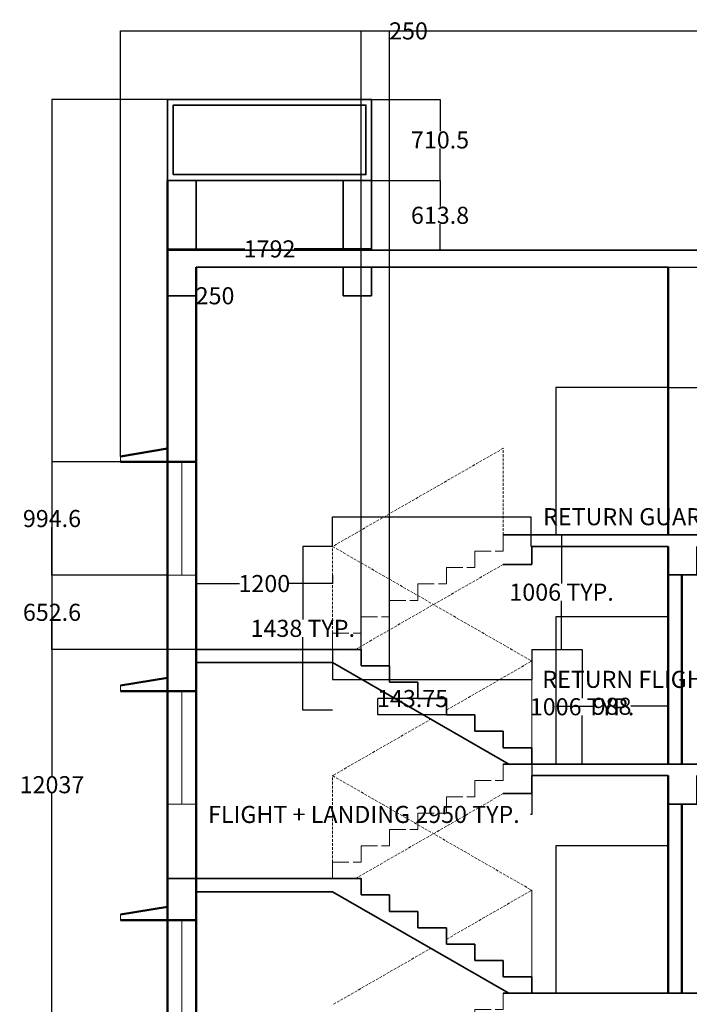
# Model space of a CAD drawing. Units: millimetres. Extents: x -1193 to 12449, y -949 to 12489.
# Tile 1 of 2: x -1193 to 4692, y 3842 to 12489. Entities that reach past the tile are written whole.
import ezdxf

# ---------------------------------------------------------------- set-up
doc = ezdxf.new("R2010")
doc.units = ezdxf.units.MM
doc.header["$LTSCALE"] = 12
doc.header["$MEASUREMENT"] = 0
doc.linetypes.add('ACAD_ISO02W100', pattern=[15, 12, -3])
doc.linetypes.add('HIDDEN', pattern=[0.375, 0.25, -0.125])
for name, color, linetype, lineweight in [('A-ANNO-DIMS', 2, 'Continuous', 18), ('A-DOOR', 3, 'Continuous', 25), ('A-FLOR', 7, 'Continuous', 35), ('A-FLOR-HRAL-BYND', 8, 'ACAD_ISO02W100', 18), ('A-FLOR-HRAL-HIDN', 8, 'HIDDEN', 18), ('A-FLOR-STRS', 7, 'Continuous', 35), ('A-FLOR-STRS-BYND', 8, 'ACAD_ISO02W100', 18), ('A-FLOR-STRS-HIDN', 8, 'HIDDEN', 18), ('A-GLAZ', 4, 'Continuous', 18), ('A-ROOF', 7, 'Continuous', 35), ('A-WALL', 7, 'Continuous', 50), ('A-WALL-BYND', 8, 'ACAD_ISO02W100', 18), ('S-BEAM', 1, 'Continuous', 35)]:
    doc.layers.add(name, color=color, linetype=linetype, lineweight=lineweight)
doc.styles.get("Standard").update_dxf_attribs({"font": 'arial.ttf'})
doc.dimstyles.get("Standard").update_dxf_attribs({"dimtxt": 150, "dimasz": 0.18, "dimexe": 0.18, "dimexo": 0.0625, "dimgap": 0.09, "dimtad": 0, "dimtih": 1, "dimtoh": 1, "dimdec": 0, "dimzin": 0, "dimdsep": 46, "dimtxsty": 'Standard', "dimcen": 0.09, "dimadec": 0, "dimazin": 0, "dimtfac": 1, "dimtdec": 0, "dimtofl": 0, "dimtmove": 0, "dimatfit": 3, "dimfxl": 1, "dimtolj": 1, "dimtzin": 0, "dimarcsym": 0})

# ---------------------------------------------------------------- blocks, each defined once
blk = doc.blocks.new('*D1')
at = {"layer": 'A-ANNO-DIMS', "color": 0, "lineweight": -2, "ltscale": 8, "transparency": 16777216}
for p, q in [((357.0112971154486, 7610.496564102366), (357.0112971154486, 7536.691782342278)), ((1557.011297115449, 7610.496564102368), (1557.011297115449, 7536.691782342278)), ((357.1912971154485, 7536.871782342278), (740.2603148507828, 7536.871782342278)), ((1556.831297115448, 7536.871782342278), (1173.762279380114, 7536.871782342278))]:
    blk.add_line(p, q, dxfattribs=at)
at = {"layer": 'A-ANNO-DIMS', "color": 0, "ltscale": 8, "transparency": 16777216}
for points in [[(357.1912971154485, 7536.901782342278), (357.1912971154485, 7536.841782342277), (357.0112971154486, 7536.871782342278)], [(1556.831297115448, 7536.901782342278), (1556.831297115448, 7536.841782342277), (1557.011297115449, 7536.871782342278)]]:
    blk.add_solid(points, dxfattribs=at)
at = {"layer": 'Defpoints', "color": 0, "ltscale": 8, "transparency": 16777216}
for p in [(357.0112971154486, 7610.559064102368), (1557.011297115449, 7610.559064102368), (1557.011297115449, 7536.871782342278)]:
    blk.add_point(p, dxfattribs=at)
at = {"layer": 'A-ANNO-DIMS', "color": 0, "ltscale": 8, "transparency": 16777216, "insert": (957.0112971154484, 7536.871782342278), "char_height": 150, "attachment_point": 5}
blk.add_mtext('\\A1;1200', dxfattribs=at)
blk = doc.blocks.new('*D2')
at = {"layer": 'A-ANNO-DIMS', "color": 0, "lineweight": -2, "ltscale": 8, "transparency": 16777216}
for p, q in [((3519.003756800259, 6598.667868016852), (3519.003756800259, 6459.014847604733)), ((4507.011297115449, 6598.667868016852), (4507.011297115449, 6459.014847604733)), ((3519.183756800259, 6459.194847604734), (3847.058045375316, 6459.194847604734)), ((4506.831297115448, 6459.194847604734), (4178.957008540391, 6459.194847604734))]:
    blk.add_line(p, q, dxfattribs=at)
at = {"layer": 'A-ANNO-DIMS', "color": 0, "ltscale": 8, "transparency": 16777216}
for points in [[(3519.183756800259, 6459.224847604733), (3519.183756800259, 6459.164847604732), (3519.003756800259, 6459.194847604734)], [(4506.831297115448, 6459.224847604733), (4506.831297115448, 6459.164847604732), (4507.011297115449, 6459.194847604734)]]:
    blk.add_solid(points, dxfattribs=at)
at = {"layer": 'Defpoints', "color": 0, "ltscale": 8, "transparency": 16777216}
for p in [(3519.003756800259, 6598.730368016852), (4507.011297115449, 6598.730368016852), (4507.011297115449, 6459.194847604734)]:
    blk.add_point(p, dxfattribs=at)
at = {"layer": 'A-ANNO-DIMS', "color": 0, "ltscale": 8, "transparency": 16777216, "insert": (4013.007526957854, 6459.194847604734), "char_height": 150, "attachment_point": 5}
blk.add_mtext('\\A1;988', dxfattribs=at)
blk = doc.blocks.new('*D6')
at = {"layer": 'A-ANNO-DIMS', "color": 0, "lineweight": -2, "ltscale": 8, "transparency": 16777216}
for p, q in [((107.0112971154485, 10064.31189252442), (107.0112971154485, 10064.42939252442)), ((107.1912971154485, 10064.24939252442), (356.8312971154485, 10064.24939252442)), ((357.0112971154486, 10064.31189252442), (357.0112971154486, 10064.42939252442)), ((357.0112971154486, 10064.24939252442), (357.1912971154486, 10064.24939252442))]:
    blk.add_line(p, q, dxfattribs=at)
at = {"layer": 'A-ANNO-DIMS', "color": 0, "ltscale": 8, "transparency": 16777216}
for points in [[(107.1912971154485, 10064.27939252442), (107.1912971154485, 10064.21939252442), (107.0112971154485, 10064.24939252442)], [(356.8312971154485, 10064.27939252442), (356.8312971154485, 10064.21939252442), (357.0112971154486, 10064.24939252442)]]:
    blk.add_solid(points, dxfattribs=at)
at = {"layer": 'Defpoints', "color": 0, "ltscale": 8, "transparency": 16777216}
for p in [(107.0112971154485, 10064.24939252442), (357.0112971154486, 10064.24939252442), (357.0112971154486, 10064.24939252442)]:
    blk.add_point(p, dxfattribs=at)
at = {"layer": 'A-ANNO-DIMS', "color": 0, "ltscale": 8, "transparency": 16777216, "insert": (524.0104922041252, 10064.24939252442), "char_height": 150, "attachment_point": 5}
blk.add_mtext('\\A1;250', dxfattribs=at)
blk = doc.blocks.new('*D7')
at = {"layer": 'A-ANNO-DIMS', "color": 0, "lineweight": -2, "ltscale": 8, "transparency": 16777216}
for p, q in [((4507.073797115451, 10464.24939252442), (5189.656778496646, 10464.24939252442)), ((5189.476778496646, 10464.24939252442), (5189.476778496646, 10464.42939252443)), ((5189.476778496646, 10464.42939252443), (5189.656778496646, 10464.42939252443)), ((5189.476778496646, 10314.42939252443), (5189.476778496646, 10464.06939252442)), ((4507.073797115451, 10314.24939252443), (5189.656778496646, 10314.24939252443))]:
    blk.add_line(p, q, dxfattribs=at)
at = {"layer": 'A-ANNO-DIMS', "color": 0, "ltscale": 8, "transparency": 16777216}
for points in [[(5189.446778496646, 10464.06939252442), (5189.506778496646, 10464.06939252442), (5189.476778496646, 10464.24939252442)], [(5189.446778496646, 10314.42939252443), (5189.506778496646, 10314.42939252443), (5189.476778496646, 10314.24939252443)]]:
    blk.add_solid(points, dxfattribs=at)
at = {"layer": 'Defpoints', "color": 0, "ltscale": 8, "transparency": 16777216}
for p in [(4507.01129711545, 10464.24939252442), (5189.476778496646, 10464.24939252442), (4507.01129711545, 10314.24939252443)]:
    blk.add_point(p, dxfattribs=at)
at = {"layer": 'A-ANNO-DIMS', "color": 0, "ltscale": 8, "transparency": 16777216, "insert": (5348.136955849991, 10464.42939252442), "char_height": 150, "attachment_point": 5}
blk.add_mtext('\\A1;150', dxfattribs=at)
blk = doc.blocks.new('STAIR-FLIGHT-LANDING-TYP')
at = {"ltscale": 8}
for p, q in [((1200, 1006.25), (-5.68e-14, 1006.25)), ((1200, 890.8972800494066), (-5.68e-14, 890.8972800494066))]:
    blk.add_line(p, q, dxfattribs=at)
for p, q in [((1450, 1006.25), (1200, 1006.25)), ((1450, 862.5), (1450, 1006.25)), ((1700, 862.5), (1450, 862.5)), ((1700, 718.75), (1700, 862.5)), ((1950, 718.75), (1700, 718.75)), ((1950, 575), (1950, 718.75)), ((2200, 575), (1950, 575)), ((2200, 431.25), (2200, 575)), ((2450, 431.25), (2200, 431.25)), ((2450, 287.5), (2450, 431.25)), ((2700, 287.5), (2450, 287.5)), ((2700, 143.75), (2700, 287.5)), ((2950, 143.75), (2700, 143.75)), ((2950, 0), (2950, 143.75))]:
    blk.add_line(p, q)
blk.add_lwpolyline([(1200, 890.8972800494066), (2749.386573998968, 0)], dxfattribs=at)
blk = doc.blocks.new('STAIR-RETURN-TYP')
for p, q in [((1500, 862.5), (1500, 1006.25)), ((1500, 1006.25), (1750, 1006.25)), ((1250, 718.75), (1250, 862.5)), ((1250, 862.5), (1500, 862.5)), ((999.9999999999995, 575), (999.9999999999995, 718.75)), ((999.9999999999995, 718.75), (1250, 718.75)), ((749.9999999999995, 431.25), (749.9999999999995, 575)), ((749.9999999999995, 575), (999.9999999999995, 575)), ((499.9999999999995, 287.5), (499.9999999999995, 431.25)), ((499.9999999999995, 431.25), (749.9999999999995, 431.25)), ((249.9999999999996, 143.75), (249.9999999999996, 287.5)), ((249.9999999999996, 287.5), (499.9999999999995, 287.5)), ((-4.547e-13, 0), (-4.547e-13, 143.75)), ((-4.547e-13, 143.75), (249.9999999999996, 143.75))]:
    blk.add_line(p, q)
blk = doc.blocks.new('DOOR-STAIR-OPENING')
at = {"ltscale": 8}
for p, q in [((988.0075403151895, 1293.961950984857), (0, 1293.961950984857)), ((0, 1293.961950984857), (0, 0))]:
    blk.add_line(p, q, dxfattribs=at)
blk = doc.blocks.new('BEAM-DROP-250x250')
for p, q in [((0, 250), (0, 0)), ((250, 0), (250, 250)), ((0, 0), (250, 0))]:
    blk.add_line(p, q)
blk = doc.blocks.new('GUARD-RETURN-TYP')
at = {"ltscale": 8}
for p, q in [((-4.547e-13, 677.0000000000045), (-4.547e-13, 1437.500000000001)), ((-4.547e-13, 1437.500000000001), (1742.461684321239, 435.5845315152882)), ((1742.461684321239, 426.9154684847135), (999.9999999999995, 0))]:
    blk.add_line(p, q, dxfattribs=at)
blk.add_arc((1739.969328699948, 431.2500000000008), 5, 299.8989018386123, 60.10109816138769, dxfattribs=at)
blk = doc.blocks.new('*D17')
at = {"layer": 'A-ANNO-DIMS', "color": 0, "lineweight": -2, "ltscale": 8, "transparency": 16777216}
for p, q in [((357.0112971154486, 5951.686892524424), (357.0112971154486, 5509.069392524423)), ((3307.011297115449, 5951.686892524424), (3307.011297115449, 5509.069392524423)), ((357.1912971154485, 5509.249392524424), (367.7330297211786, 5509.249392524424)), ((3306.831297115449, 5509.249392524424), (3296.289564509719, 5509.249392524424))]:
    blk.add_line(p, q, dxfattribs=at)
at = {"layer": 'A-ANNO-DIMS', "color": 0, "ltscale": 8, "transparency": 16777216}
for points in [[(357.1912971154485, 5509.279392524424), (357.1912971154485, 5509.219392524425), (357.0112971154486, 5509.249392524424)], [(3306.831297115449, 5509.279392524424), (3306.831297115449, 5509.219392524425), (3307.011297115449, 5509.249392524424)]]:
    blk.add_solid(points, dxfattribs=at)
at = {"layer": 'Defpoints', "color": 0, "ltscale": 8, "transparency": 16777216}
for p in [(357.0112971154486, 5951.749392524424), (3307.011297115449, 5951.749392524424), (3307.011297115449, 5509.249392524424)]:
    blk.add_point(p, dxfattribs=at)
at = {"layer": 'A-ANNO-DIMS', "color": 0, "ltscale": 8, "transparency": 16777216, "insert": (1832.011297115449, 5509.249392524424), "char_height": 150, "attachment_point": 5}
blk.add_mtext('\\A1;FLIGHT + LANDING 2950 TYP.', dxfattribs=at)
blk = doc.blocks.new('*D18')
at = {"layer": 'A-ANNO-DIMS', "color": 0, "lineweight": -2, "ltscale": 8, "transparency": 16777216}
for p, q in [((3307.073797115451, 6957.999392524428), (3749.691297115453, 6957.999392524428)), ((3749.511297115453, 6957.819392524427), (3749.511297115453, 6531.550340682682)), ((3749.511297115453, 5951.929392524426), (3749.511297115453, 6378.198444366174)), ((3307.073797115451, 5951.749392524426), (3749.691297115453, 5951.749392524426))]:
    blk.add_line(p, q, dxfattribs=at)
at = {"layer": 'A-ANNO-DIMS', "color": 0, "ltscale": 8, "transparency": 16777216}
for points in [[(3749.481297115452, 6957.819392524427), (3749.541297115453, 6957.819392524427), (3749.511297115453, 6957.999392524428)], [(3749.481297115452, 5951.929392524426), (3749.541297115453, 5951.929392524426), (3749.511297115453, 5951.749392524426)]]:
    blk.add_solid(points, dxfattribs=at)
at = {"layer": 'Defpoints', "color": 0, "ltscale": 8, "transparency": 16777216}
for p in [(3307.01129711545, 6957.999392524428), (3749.511297115453, 6957.999392524428), (3307.01129711545, 5951.749392524426)]:
    blk.add_point(p, dxfattribs=at)
at = {"layer": 'A-ANNO-DIMS', "color": 0, "ltscale": 8, "transparency": 16777216, "insert": (3749.511297115454, 6454.874392524425), "char_height": 150, "attachment_point": 5}
blk.add_mtext('\\A1;1006 TYP.', dxfattribs=at)
blk = doc.blocks.new('*D19')
at = {"layer": 'A-ANNO-DIMS', "color": 0, "lineweight": -2, "ltscale": 8, "transparency": 16777216}
for p, q in [((1557.011297115448, 6957.936892524424), (1557.011297115448, 6695.319392524424)), ((3307.01129711545, 6957.936892524424), (3307.01129711545, 6695.319392524424)), ((1557.191297115448, 6695.499392524424), (3306.831297115449, 6695.499392524424)), ((3307.01129711545, 6695.499392524424), (3307.19129711545, 6695.499392524424))]:
    blk.add_line(p, q, dxfattribs=at)
at = {"layer": 'A-ANNO-DIMS', "color": 0, "ltscale": 8, "transparency": 16777216}
for points in [[(1557.191297115448, 6695.529392524425), (1557.191297115448, 6695.469392524424), (1557.011297115448, 6695.499392524424)], [(3306.831297115449, 6695.529392524425), (3306.831297115449, 6695.469392524424), (3307.01129711545, 6695.499392524424)]]:
    blk.add_solid(points, dxfattribs=at)
at = {"layer": 'Defpoints', "color": 0, "ltscale": 8, "transparency": 16777216}
for p in [(1557.011297115448, 6957.999392524424), (3307.01129711545, 6957.999392524424), (3307.01129711545, 6695.499392524424)]:
    blk.add_point(p, dxfattribs=at)
at = {"layer": 'A-ANNO-DIMS', "color": 0, "ltscale": 8, "transparency": 16777216, "insert": (4652.318814168655, 6695.499392524424), "char_height": 150, "attachment_point": 5}
blk.add_mtext('\\A1;RETURN FLIGHT 1750 TYP.', dxfattribs=at)
blk = doc.blocks.new('*D20')
at = {"layer": 'A-ANNO-DIMS', "color": 0, "lineweight": -2, "ltscale": 8, "transparency": 16777216}
for p, q in [((3307.073797115451, 7964.249392524428), (3569.691297115453, 7964.249392524428)), ((3569.511297115453, 7964.069392524428), (3569.511297115453, 7537.800340682682)), ((3569.511297115453, 6958.179392524428), (3569.511297115453, 7384.448444366174)), ((3307.073797115451, 6957.999392524428), (3569.691297115453, 6957.999392524428))]:
    blk.add_line(p, q, dxfattribs=at)
at = {"layer": 'A-ANNO-DIMS', "color": 0, "ltscale": 8, "transparency": 16777216}
for points in [[(3569.481297115453, 7964.069392524428), (3569.541297115453, 7964.069392524428), (3569.511297115453, 7964.249392524428)], [(3569.481297115453, 6958.179392524428), (3569.541297115453, 6958.179392524428), (3569.511297115453, 6957.999392524428)]]:
    blk.add_solid(points, dxfattribs=at)
at = {"layer": 'Defpoints', "color": 0, "ltscale": 8, "transparency": 16777216}
for p in [(3307.011297115451, 7964.249392524428), (3569.511297115453, 7964.249392524428), (3307.011297115451, 6957.999392524428)]:
    blk.add_point(p, dxfattribs=at)
at = {"layer": 'A-ANNO-DIMS', "color": 0, "ltscale": 8, "transparency": 16777216, "insert": (3569.511297115454, 7461.124392524425), "char_height": 150, "attachment_point": 5}
blk.add_mtext('\\A1;1006 TYP.', dxfattribs=at)
blk = doc.blocks.new('*D21')
at = {"layer": 'A-ANNO-DIMS', "color": 0, "lineweight": -2, "ltscale": 8, "transparency": 16777216}
for p, q in [((1557.011297115448, 7862.311892524418), (1557.011297115448, 8124.17479182941)), ((1557.191297115448, 8123.99479182941), (3301.800625815397, 8123.99479182941)), ((3301.980625815397, 7862.311892524418), (3301.980625815397, 8124.17479182941)), ((3301.980625815397, 8123.99479182941), (3302.160625815397, 8123.99479182941))]:
    blk.add_line(p, q, dxfattribs=at)
at = {"layer": 'A-ANNO-DIMS', "color": 0, "ltscale": 8, "transparency": 16777216}
for points in [[(1557.191297115448, 8124.024791829411), (1557.191297115448, 8123.964791829411), (1557.011297115448, 8123.99479182941)], [(3301.800625815397, 8124.024791829411), (3301.800625815397, 8123.964791829411), (3301.980625815397, 8123.99479182941)]]:
    blk.add_solid(points, dxfattribs=at)
at = {"layer": 'Defpoints', "color": 0, "ltscale": 8, "transparency": 16777216}
for p in [(3301.980625815397, 8123.99479182941), (1557.011297115448, 7862.249392524418), (3301.980625815397, 7862.249392524418)]:
    blk.add_point(p, dxfattribs=at)
at = {"layer": 'A-ANNO-DIMS', "color": 0, "ltscale": 8, "transparency": 16777216, "insert": (4653.120339321535, 8123.99479182941), "char_height": 150, "attachment_point": 5}
blk.add_mtext('\\A1;RETURN GUARD 1745 TYP.', dxfattribs=at)
blk = doc.blocks.new('*D22')
at = {"layer": 'A-ANNO-DIMS', "color": 0, "lineweight": -2, "ltscale": 8, "transparency": 16777216}
for p, q in [((1556.948797115449, 7862.249392524423), (1295.085897810457, 7862.249392524423)), ((1295.265897810457, 7862.069392524422), (1295.265897810457, 7220.226500300682)), ((1295.265897810457, 6424.929392524422), (1295.265897810457, 7066.77228474816)), ((1556.948797115449, 6424.749392524422), (1295.085897810457, 6424.749392524422))]:
    blk.add_line(p, q, dxfattribs=at)
at = {"layer": 'A-ANNO-DIMS', "color": 0, "ltscale": 8, "transparency": 16777216}
for points in [[(1295.235897810457, 7862.069392524422), (1295.295897810457, 7862.069392524422), (1295.265897810457, 7862.249392524423)], [(1295.235897810457, 6424.929392524422), (1295.295897810457, 6424.929392524422), (1295.265897810457, 6424.749392524422)]]:
    blk.add_solid(points, dxfattribs=at)
at = {"layer": 'Defpoints', "color": 0, "ltscale": 8, "transparency": 16777216}
for p in [(1295.265897810457, 7862.249392524423), (1557.011297115449, 7862.249392524423), (1557.011297115449, 6424.749392524422)]:
    blk.add_point(p, dxfattribs=at)
at = {"layer": 'A-ANNO-DIMS', "color": 0, "ltscale": 8, "transparency": 16777216, "insert": (1295.265897810459, 7143.49939252442), "char_height": 150, "attachment_point": 5}
blk.add_mtext('\\A1;1438 TYP.', dxfattribs=at)
blk = doc.blocks.new('*D27')
at = {"layer": 'A-ANNO-DIMS', "color": 0, "lineweight": -2, "ltscale": 8, "transparency": 16777216}
for p, q in [((-307.014113, 8654.059893999998), (-307.0141129999998, 12390.66548)), ((-306.8341129999998, 12390.48548), (4949.545781004093, 12390.48548)), ((10754.946057, 12390.48548), (5498.566162995907, 12390.48548)), ((10755.126057, 7964.311893), (10755.126057, 12390.66548))]:
    blk.add_line(p, q, dxfattribs=at)
at = {"layer": 'A-ANNO-DIMS', "color": 0, "ltscale": 8, "transparency": 16777216}
for points in [[(-306.8341129999998, 12390.51548), (-306.8341129999998, 12390.45548), (-307.0141129999998, 12390.48548)], [(10754.946057, 12390.51548), (10754.946057, 12390.45548), (10755.126057, 12390.48548)]]:
    blk.add_solid(points, dxfattribs=at)
at = {"layer": 'Defpoints', "color": 0, "ltscale": 8, "transparency": 16777216}
for p in [(10755.126057, 12390.48548), (-307.014113, 8653.997393999998), (10755.126057, 7964.249393)]:
    blk.add_point(p, dxfattribs=at)
at = {"layer": 'A-ANNO-DIMS', "color": 0, "ltscale": 8, "transparency": 16777216, "insert": (5224.055972, 12390.48548), "char_height": 150, "attachment_point": 5}
blk.add_mtext('\\A1;11062', dxfattribs=at)
blk = doc.blocks.new('*D28')
at = {"layer": 'A-ANNO-DIMS', "color": 0, "lineweight": -2, "ltscale": 8, "transparency": 16777216}
for p, q in [((106.948797, 11788.48548), (-909.1941130000021, 11788.48548)), ((-909.0141130000022, 11788.30548), (-909.0141130000007, 5846.844544276263)), ((-909.0141129999995, -248.0706070000003), (-909.0141130000007, 5693.39032872374)), ((106.948797, -248.2506070000001), (-909.1941129999994, -248.2506070000003))]:
    blk.add_line(p, q, dxfattribs=at)
at = {"layer": 'A-ANNO-DIMS', "color": 0, "ltscale": 8, "transparency": 16777216}
for points in [[(-909.0441130000021, 11788.30548), (-908.9841130000023, 11788.30548), (-909.0141130000022, 11788.48548)], [(-909.0441129999996, -248.0706070000003), (-908.9841129999996, -248.0706070000003), (-909.0141129999995, -248.2506070000003)]]:
    blk.add_solid(points, dxfattribs=at)
at = {"layer": 'Defpoints', "color": 0, "ltscale": 8, "transparency": 16777216}
for p in [(-909.0141130000022, 11788.48548), (107.011297, 11788.48548), (107.011297, -248.2506070000001)]:
    blk.add_point(p, dxfattribs=at)
at = {"layer": 'A-ANNO-DIMS', "color": 0, "ltscale": 8, "transparency": 16777216, "insert": (-909.014112999999, 5770.117436500001), "char_height": 150, "attachment_point": 5}
blk.add_mtext('\\A1;12037', dxfattribs=at)
blk = doc.blocks.new('*D41')
at = {"layer": 'A-ANNO-DIMS', "color": 0, "lineweight": -2, "ltscale": 8, "transparency": 16777216}
for p, q in [((1899.223943000001, 11078.003928), (2501.341443000002, 11078.003928)), ((2501.161443000002, 11077.823928), (2501.161443000002, 10847.85376827626)), ((2501.161443000002, 10464.429393), (2501.161443000002, 10694.39955272374)), ((1899.223943000001, 10464.249393), (2501.341443000002, 10464.249393))]:
    blk.add_line(p, q, dxfattribs=at)
at = {"layer": 'A-ANNO-DIMS', "color": 0, "ltscale": 8, "transparency": 16777216}
for points in [[(2501.131443000002, 11077.823928), (2501.191443000002, 11077.823928), (2501.161443000002, 11078.003928)], [(2501.131443000002, 10464.429393), (2501.191443000002, 10464.429393), (2501.161443000002, 10464.249393)]]:
    blk.add_solid(points, dxfattribs=at)
at = {"layer": 'Defpoints', "color": 0, "ltscale": 8, "transparency": 16777216}
for p in [(1899.161443000001, 11078.003928), (1899.161443000001, 10464.249393), (2501.161443000002, 10464.249393)]:
    blk.add_point(p, dxfattribs=at)
at = {"layer": 'A-ANNO-DIMS', "color": 0, "ltscale": 8, "transparency": 16777216, "insert": (2501.161443000004, 10771.1266605), "char_height": 150, "attachment_point": 5}
blk.add_mtext('\\A1;613.8', dxfattribs=at)
blk = doc.blocks.new('*D42')
at = {"layer": 'A-ANNO-DIMS', "color": 0, "lineweight": -2, "ltscale": 8, "transparency": 16777216}
for p, q in [((1899.223943000001, 11788.48548), (2501.341443000002, 11788.48548)), ((2501.161443000002, 11788.30548), (2501.161443000002, 11509.92065215825)), ((2501.161443000003, 11078.183928), (2501.161443000002, 11356.56875584175)), ((1899.223943000001, 11078.003928), (2501.341443000002, 11078.003928))]:
    blk.add_line(p, q, dxfattribs=at)
at = {"layer": 'A-ANNO-DIMS', "color": 0, "ltscale": 8, "transparency": 16777216}
for points in [[(2501.131443000002, 11788.30548), (2501.191443000002, 11788.30548), (2501.161443000002, 11788.48548)], [(2501.131443000002, 11078.183928), (2501.191443000003, 11078.183928), (2501.161443000003, 11078.003928)]]:
    blk.add_solid(points, dxfattribs=at)
at = {"layer": 'Defpoints', "color": 0, "ltscale": 8, "transparency": 16777216}
for p in [(1899.161443000001, 11788.48548), (1899.161443000001, 11078.003928), (2501.161443000003, 11078.003928)]:
    blk.add_point(p, dxfattribs=at)
at = {"layer": 'A-ANNO-DIMS', "color": 0, "ltscale": 8, "transparency": 16777216, "insert": (2501.161443000005, 11433.244704), "char_height": 150, "attachment_point": 5}
blk.add_mtext('\\A1;710.5', dxfattribs=at)
blk = doc.blocks.new('*D43')
at = {"layer": 'A-ANNO-DIMS', "color": 0, "lineweight": -2, "ltscale": 8, "transparency": 16777216}
for p, q in [((107.011297, 11077.941428), (107.0112969999999, 10475.823928)), ((1899.161443, 11077.941428), (1899.161443, 10475.823928)), ((107.1912969999999, 10476.003928), (786.8469839154161, 10476.003928)), ((1898.981443, 10476.003928), (1219.325756084584, 10476.003928))]:
    blk.add_line(p, q, dxfattribs=at)
at = {"layer": 'A-ANNO-DIMS', "color": 0, "ltscale": 8, "transparency": 16777216}
for points in [[(107.1912969999999, 10476.033928), (107.1912969999999, 10475.973928), (107.0112969999999, 10476.003928)], [(1898.981443, 10476.033928), (1898.981443, 10475.973928), (1899.161443, 10476.003928)]]:
    blk.add_solid(points, dxfattribs=at)
at = {"layer": 'Defpoints', "color": 0, "ltscale": 8, "transparency": 16777216}
for p in [(107.011297, 11078.003928), (1899.161443, 11078.003928), (107.0112969999999, 10476.003928)]:
    blk.add_point(p, dxfattribs=at)
at = {"layer": 'A-ANNO-DIMS', "color": 0, "ltscale": 8, "transparency": 16777216, "insert": (1003.08637, 10476.003928), "char_height": 150, "attachment_point": 5}
blk.add_mtext('\\A1;1792', dxfattribs=at)
blk = doc.blocks.new('*D44')
at = {"layer": 'A-ANNO-DIMS', "color": 0, "lineweight": -2, "ltscale": 8, "transparency": 16777216}
for p, q in [((4507.073797000002, 9258.211344000001), (11357.306057, 9258.211344000001)), ((11357.126057, 9258.031344000003), (11357.126057, 8687.906316658258)), ((11357.126057, 7964.429393000006), (11357.126057, 8534.55442034175)), ((4507.073797000002, 7964.249393000004), (11357.306057, 7964.249393000006))]:
    blk.add_line(p, q, dxfattribs=at)
at = {"layer": 'A-ANNO-DIMS', "color": 0, "ltscale": 8, "transparency": 16777216}
for points in [[(11357.096057, 9258.031344000003), (11357.15605700001, 9258.031344000003), (11357.126057, 9258.211344000001)], [(11357.096057, 7964.429393000006), (11357.15605700001, 7964.429393000006), (11357.126057, 7964.249393000006)]]:
    blk.add_solid(points, dxfattribs=at)
at = {"layer": 'Defpoints', "color": 0, "ltscale": 8, "transparency": 16777216}
for p in [(4507.011297000001, 9258.211344000001), (11357.126057, 9258.211344000001), (4507.011297000001, 7964.249393000004)]:
    blk.add_point(p, dxfattribs=at)
at = {"layer": 'A-ANNO-DIMS', "color": 0, "ltscale": 8, "transparency": 16777216, "insert": (11357.126057, 8611.2303685), "char_height": 150, "attachment_point": 5}
blk.add_mtext('\\A1;1294', dxfattribs=at)
blk = doc.blocks.new('*D45')
at = {"layer": 'A-ANNO-DIMS', "color": 0, "lineweight": -2, "ltscale": 8, "transparency": 16777216}
for p, q in [((106.948797, 8605.146673000003), (-909.1941130000009, 8605.146673000003)), ((-909.0141130000009, 8604.966673000003), (-909.0141130000007, 8184.528816658257)), ((-909.0141130000007, 7610.739064000004), (-909.0141130000007, 8031.176920341749)), ((106.948797, 7610.559064000004), (-909.1941130000007, 7610.559064000004))]:
    blk.add_line(p, q, dxfattribs=at)
at = {"layer": 'A-ANNO-DIMS', "color": 0, "ltscale": 8, "transparency": 16777216}
for points in [[(-909.044113000001, 8604.966673000003), (-908.984113000001, 8604.966673000003), (-909.0141130000009, 8605.146673000003)], [(-909.0441130000007, 7610.739064000004), (-908.9841130000008, 7610.739064000004), (-909.0141130000007, 7610.559064000004)]]:
    blk.add_solid(points, dxfattribs=at)
at = {"layer": 'Defpoints', "color": 0, "ltscale": 8, "transparency": 16777216}
for p in [(-909.0141130000009, 8605.146673000003), (107.011297, 8605.146673000003), (107.011297, 7610.559064000004)]:
    blk.add_point(p, dxfattribs=at)
at = {"layer": 'A-ANNO-DIMS', "color": 0, "ltscale": 8, "transparency": 16777216, "insert": (-909.0141129999982, 8107.852868500001), "char_height": 150, "attachment_point": 5}
blk.add_mtext('\\A1;994.6', dxfattribs=at)
blk = doc.blocks.new('*D46')
at = {"layer": 'A-ANNO-DIMS', "color": 0, "lineweight": -2, "ltscale": 8, "transparency": 16777216}
for p, q in [((106.948797, 7610.559064000004), (-909.1941130000009, 7610.559064000004)), ((-909.0141130000009, 7610.379064000004), (-909.0141130000007, 7360.955176658257)), ((-909.0141130000007, 6958.179393000005), (-909.0141130000007, 7207.603280341749)), ((356.9487970000001, 6957.999393000005), (-909.1941130000009, 6957.999393000005))]:
    blk.add_line(p, q, dxfattribs=at)
at = {"layer": 'A-ANNO-DIMS', "color": 0, "ltscale": 8, "transparency": 16777216}
for points in [[(-909.044113000001, 7610.379064000004), (-908.984113000001, 7610.379064000004), (-909.0141130000009, 7610.559064000004)], [(-909.044113000001, 6958.179393000005), (-908.9841130000008, 6958.179393000005), (-909.0141130000007, 6957.999393000005)]]:
    blk.add_solid(points, dxfattribs=at)
at = {"layer": 'Defpoints', "color": 0, "ltscale": 8, "transparency": 16777216}
for p in [(-909.0141130000009, 7610.559064000004), (107.011297, 7610.559064000004), (357.0112970000001, 6957.999393000005)]:
    blk.add_point(p, dxfattribs=at)
at = {"layer": 'A-ANNO-DIMS', "color": 0, "ltscale": 8, "transparency": 16777216, "insert": (-909.0141129999986, 7284.279228500001), "char_height": 150, "attachment_point": 5}
blk.add_mtext('\\A1;652.6', dxfattribs=at)
blk = doc.blocks.new('*D47')
at = {"layer": 'A-ANNO-DIMS', "color": 0, "lineweight": -2, "ltscale": 8, "transparency": 16777216}
for p, q in [((1807.011297, 6814.311893), (1807.011297, 12390.66548)), ((1807.191297000001, 12390.48548), (2056.831297000001, 12390.48548)), ((2057.011297, 6814.311893), (2057.011297, 12390.66548)), ((2057.011297, 12390.48548), (2057.191297000001, 12390.48548))]:
    blk.add_line(p, q, dxfattribs=at)
at = {"layer": 'A-ANNO-DIMS', "color": 0, "ltscale": 8, "transparency": 16777216}
for points in [[(1807.191297000001, 12390.51548), (1807.191297000001, 12390.45548), (1807.011297, 12390.48548)], [(2056.831297000001, 12390.51548), (2056.831297000001, 12390.45548), (2057.011297, 12390.48548)]]:
    blk.add_solid(points, dxfattribs=at)
at = {"layer": 'Defpoints', "color": 0, "ltscale": 8, "transparency": 16777216}
for p in [(2057.011297, 12390.48548), (1807.011297, 6814.249393), (2057.011297, 6814.249393)]:
    blk.add_point(p, dxfattribs=at)
at = {"layer": 'A-ANNO-DIMS', "color": 0, "ltscale": 8, "transparency": 16777216, "insert": (2224.010492088677, 12390.48548), "char_height": 150, "attachment_point": 5}
blk.add_mtext('\\A1;250', dxfattribs=at)
blk = doc.blocks.new('*D48')
at = {"layer": 'A-ANNO-DIMS', "color": 0, "lineweight": -2, "ltscale": 8, "transparency": 16777216}
for p, q in [((2556.948797000001, 6526.749393000004), (1954.831297000002, 6526.749393000002)), ((1955.011297000002, 6526.749393000002), (1955.011297000002, 6526.929393000003)), ((1955.011297000002, 6526.929393000003), (1955.191297000002, 6526.929393000003)), ((1955.011297000002, 6383.179393000003), (1955.011297000002, 6526.569393000002)), ((2556.948797000001, 6382.999393000003), (1954.831297000002, 6382.999393000003))]:
    blk.add_line(p, q, dxfattribs=at)
at = {"layer": 'A-ANNO-DIMS', "color": 0, "ltscale": 8, "transparency": 16777216}
for points in [[(1954.981297000002, 6526.569393000002), (1955.041297000002, 6526.569393000002), (1955.011297000002, 6526.749393000002)], [(1954.981297000002, 6383.179393000003), (1955.041297000002, 6383.179393000003), (1955.011297000002, 6382.999393000003)]]:
    blk.add_solid(points, dxfattribs=at)
at = {"layer": 'Defpoints', "color": 0, "ltscale": 8, "transparency": 16777216}
for p in [(1955.011297000002, 6526.749393000002), (2557.011297000001, 6526.749393000004), (2557.011297000001, 6382.999393000003)]:
    blk.add_point(p, dxfattribs=at)
at = {"layer": 'A-ANNO-DIMS', "color": 0, "ltscale": 8, "transparency": 16777216, "insert": (2260.141460710781, 6526.929393000002), "char_height": 150, "attachment_point": 5}
blk.add_mtext('\\A1;143.75', dxfattribs=at)

msp = doc.modelspace()

# ---------------------------------------------------------------- linework, layer by layer
at = {"layer": 'A-FLOR', "ltscale": 8}
for p, q in [((3057.011297115449, 5951.749392524424), (10755.12605663696, 5951.749392524424)), ((3307.011297115448, 5849.749392524423), (4507.011297115449, 5849.749392524423)), ((3057.011297115449, 3939.249392524423), (10755.12605663696, 3939.249392524423))]:
    msp.add_line(p, q, dxfattribs=at)
at = {"layer": 'A-FLOR-HRAL-BYND', "ltscale": 8}
for p, q in [((3307.011297115449, 6095.499392524423), (3307.011297115449, 6855.99939252442)), ((3307.011297115449, 4082.999392524423), (3307.011297115449, 4843.49939252442))]:
    msp.add_line(p, q, dxfattribs=at)
at = {"layer": 'A-FLOR-HRAL-HIDN', "ltscale": 8}
for p, q in [((3057.011297115449, 8724.749392524422), (1557.011297115449, 7862.24939252442)), ((3057.011297115449, 7964.249392524424), (3057.011297115449, 8724.749392524422)), ((1564.54961279421, 5854.083924039708), (2420.40023628885, 6346.198032549124)), ((1564.54961279421, 3841.583924039707), (2420.40023628885, 4333.698032549124))]:
    msp.add_line(p, q, dxfattribs=at)
at = {"layer": 'A-FLOR-STRS', "ltscale": 8}
for p, q in [((3307.011297115449, 7704.74667257383), (3307.011297115448, 7862.249392524424)), ((3057.011297115449, 7704.74667257383), (3307.011297115449, 7704.74667257383)), ((3307.011297115449, 5692.24667257383), (3307.011297115448, 5849.749392524423)), ((3057.011297115449, 5692.24667257383), (3307.011297115449, 5692.24667257383)), ((357.0112971154486, 4945.499392524424), (107.0112971154485, 4945.499392524424))]:
    msp.add_line(p, q, dxfattribs=at)
at = {"layer": 'A-FLOR-STRS-HIDN', "ltscale": 8}
for points in [[(3057.011297115449, 7705.146672573831), (1757.62472311648, 6957.999392524424)], [(3057.011297115449, 5692.64667257383), (1757.62472311648, 4945.499392524424)]]:
    msp.add_lwpolyline(points, dxfattribs=at)
at = {"layer": 'A-GLAZ', "ltscale": 8}
for p, q in [((232.0112971154486, 7610.559064102368), (232.0112971154486, 8605.146672573832)), ((232.0112971154486, 5598.059064102367), (232.0112971154486, 6592.646672573831)), ((232.0112971154486, 3585.559064102367), (232.0112971154486, 4580.14667257383))]:
    msp.add_line(p, q, dxfattribs=at)
at = {"layer": 'A-ROOF', "ltscale": 8}
for p, q in [((1649.161443254372, 11078.003927741), (107.0112971154485, 11078.003927741)), ((357.0112971154484, 11078.003927741), (357.0112971154485, 10464.24939252442)), ((1899.161443254372, 11078.003927741), (1649.161443254372, 11078.003927741)), ((1649.161443254372, 11078.003927741), (1649.161443254372, 10464.24939252442)), ((1899.161443254372, 10464.24939252442), (1899.161443254372, 11078.003927741)), ((4757.011297115449, 10464.24939252442), (107.0112971154485, 10464.24939252442)), ((4507.011297115449, 10314.24939252442), (357.0112971154486, 10314.24939252442)), ((3057.011297115449, 7964.249392524424), (10755.12605663696, 7964.249392524424)), ((3307.011297115448, 7862.249392524424), (4507.011297115449, 7862.249392524424))]:
    msp.add_line(p, q, dxfattribs=at)
for points in [[(107.0112971154485, 11078.003927741), (1899.161443254372, 11078.003927741), (1899.161443254372, 11788.48548038965), (107.0112971154485, 11788.48548038965)], [(157.0112971154485, 11128.003927741), (1849.161443254372, 11128.003927741), (1849.161443254372, 11738.48548038965), (157.0112971154485, 11738.48548038965)]]:
    msp.add_lwpolyline(points, close=True, dxfattribs=at)
at = {"layer": 'A-WALL', "ltscale": 8}
for p, q in [((107.0112971154485, 11078.003927741), (107.0112971154486, 6710.23503040228)), ((357.0112971154486, 6957.999392524424), (357.0112971154485, 10314.24939252442)), ((4507.011297115449, 7964.249392524424), (4507.011297115449, 10314.24939252442)), ((-307.0141126089075, 8653.99739442215), (107.0112971154485, 8722.73503040228)), ((107.0112971154485, 8605.146672573832), (-307.0141126089075, 8605.146672573832)), ((357.0112971154486, 8605.146672573832), (107.0112971154485, 8605.146672573832)), ((4507.011297115449, 5951.749392524424), (4507.011297115449, 7862.249392524424)), ((4627.011297115449, 5951.749392524424), (4627.011297115449, 7612.249392524424)), ((-307.0141126089075, 6641.497394422149), (107.0112971154485, 6710.23503040228)), ((107.0112971154485, 6592.646672573831), (-307.0141126089075, 6592.646672573831)), ((357.0112971154486, 6592.646672573831), (107.0112971154485, 6592.646672573831)), ((4507.011297115449, 3939.249392524424), (4507.011297115449, 5849.749392524423)), ((4627.011297115449, 3939.249392524424), (4627.011297115449, 5599.749392524423)), ((-307.0141126089075, 4628.997394422149), (107.0112971154485, 4697.73503040228)), ((107.0112971154485, 4580.14667257383), (-307.0141126089075, 4580.14667257383)), ((357.0112971154486, 4580.14667257383), (107.0112971154485, 4580.14667257383))]:
    msp.add_line(p, q, dxfattribs=at)
at = {"layer": 'A-WALL'}
for p, q in [((357.0112971154486, 1.749392524423001), (357.0112971154486, 6957.999392524424)), ((107.0112971154485, 1.749392524423001), (107.0112971154486, 6710.235030402279))]:
    msp.add_line(p, q, dxfattribs=at)
at = {"layer": 'A-WALL-BYND', "ltscale": 8}
for p, q in [((-307.0141126089075, 8653.99739442215), (-307.0141126089075, 8605.146672573832)), ((357.0112971154487, 7610.559064102368), (107.0112971154485, 7610.559064102368)), ((-307.0141126089075, 6641.497394422149), (-307.0141126089075, 6592.646672573831)), ((357.0112971154487, 5598.059064102367), (107.0112971154485, 5598.059064102367)), ((-307.0141126089075, 4628.997394422149), (-307.0141126089075, 4580.14667257383))]:
    msp.add_line(p, q, dxfattribs=at)
at = {"layer": 'S-BEAM', "ltscale": 8}
for p, q in [((357.0112971154485, 10314.24939252442), (357.0112971154485, 10064.24939252442)), ((357.0112971154486, 10064.24939252442), (107.0112971154485, 10064.24939252442))]:
    msp.add_line(p, q, dxfattribs=at)

# ---------------------------------------------------------------- block references
at = {"layer": 'A-DOOR'}
for p in [(3519.003756800259, 7964.249392524424), (3519.003756800259, 5951.749392524422), (3519.003756800259, 3939.249392524422)]:
    msp.add_blockref('DOOR-STAIR-OPENING', p, dxfattribs=at)
at = {"layer": 'A-FLOR-HRAL-HIDN'}
for p in [(1557.011297115449, 6424.749392524418), (1557.011297115449, 4412.249392524419)]:
    msp.add_blockref('GUARD-RETURN-TYP', p, dxfattribs=at)
at = {"layer": 'A-FLOR-STRS'}
for p in [(357.0112971154486, 5951.749392524424), (357.0112971154487, 3939.249392524424)]:
    msp.add_blockref('STAIR-FLIGHT-LANDING-TYP', p, dxfattribs=at)
at = {"layer": 'A-FLOR-STRS-BYND'}
for p in [(1557.011297115449, 6957.999392524424), (1557.011297115449, 4945.499392524424), (1557.011297115449, 2932.999392524423)]:
    msp.add_blockref('STAIR-RETURN-TYP', p, dxfattribs=at)
at = {"layer": 'S-BEAM'}
for p in [(1649.161443254371, 10064.24939252442), (4507.011297115449, 7612.249392524424), (4507.011297115449, 5599.749392524423)]:
    msp.add_blockref('BEAM-DROP-250x250', p, dxfattribs=at)

# ---------------------------------------------------------------- dimensions: what is measured, and where the dimension line sits
at = {"layer": 'A-ANNO-DIMS', "ltscale": 8}
for base, p1, p2, picture, middle in [((10755.126057, 12390.48548), (-307.014113, 8653.997393999998), (10755.126057, 7964.249393), '*D27', (5224.055972, 12390.48548)), ((2057.011297, 12390.48548), (1807.011297, 6814.249393), (2057.011297, 6814.249393), '*D47', (2224.010492088677, 12390.48548))]:
    dim = msp.add_linear_dim(base=base, p1=p1, p2=p2, dimstyle='Standard', override={"dimdec": 0, "dimlfac": 1, "dimrnd": 0, "dimzin": 0, "dimdsep": 46, "dimlunit": 2}, dxfattribs=at)
    dim.commit()
    dim.dimension.update_dxf_attribs({"geometry": picture, "text_midpoint": middle})
for base, p1, p2, angle, override, picture, middle in [((-909.0141130000022, 11788.48548), (107.011297, -248.250607), (107.011297, 11788.48548), 90, {"dimdec": 0, "dimlfac": 1, "dimrnd": 0, "dimzin": 0, "dimdsep": 46, "dimlunit": 2}, '*D28', (-909.014112999999, 5770.117436500001)), ((2501.161443000003, 11078.003928), (1899.161443, 11788.48548), (1899.161443, 11078.003928), 270, {"dimdec": 1, "dimlfac": 1, "dimrnd": 0, "dimzin": 0, "dimdsep": 46, "dimlunit": 2}, '*D42', (2501.161443000005, 11433.244704)), ((107.0112969999999, 10476.003928), (1899.161443, 11078.003928), (107.011297, 11078.003928), 180, {"dimdec": 0, "dimlfac": 1, "dimrnd": 0, "dimzin": 0, "dimdsep": 46, "dimlunit": 2}, '*D43', (1003.08637, 10476.003928)), ((2501.161443000002, 10464.249393), (1899.161443, 11078.003928), (1899.161443, 10464.249393), 270, {"dimdec": 1, "dimlfac": 1, "dimrnd": 0, "dimzin": 0, "dimdsep": 46, "dimlunit": 2}, '*D41', (2501.161443000004, 10771.1266605)), ((11357.126057, 9258.211344000001), (4507.011297, 7964.249393), (4507.011297, 9258.211344000001), 90, {"dimdec": 0, "dimlfac": 1, "dimrnd": 0, "dimzin": 0, "dimdsep": 46, "dimlunit": 2}, '*D44', (11357.126057, 8611.2303685)), ((-909.0141130000009, 8605.146673000003), (107.011297, 7610.559064), (107.011297, 8605.146673), 90, {"dimdec": 1, "dimlfac": 1, "dimrnd": 0, "dimzin": 0, "dimdsep": 46, "dimlunit": 2}, '*D45', (-909.0141129999982, 8107.852868500001)), ((-909.0141130000009, 7610.559064000004), (357.011297, 6957.999393), (107.011297, 7610.559064), 90, {"dimdec": 1, "dimlfac": 1, "dimrnd": 0, "dimzin": 0, "dimdsep": 46, "dimlunit": 2}, '*D46', (-909.0141129999986, 7284.279228500001)), ((1955.011297000002, 6526.749393000002), (2557.011297, 6382.999393), (2557.011297, 6526.749393), 90, {"dimdec": 2, "dimlfac": 1, "dimrnd": 0, "dimzin": 0, "dimdsep": 46, "dimlunit": 2}, '*D48', (2260.141460710781, 6526.929393000002))]:
    dim = msp.add_linear_dim(base=base, p1=p1, p2=p2, angle=angle, dimstyle='Standard', override=override, dxfattribs=at)
    dim.commit()
    dim.dimension.update_dxf_attribs({"geometry": picture, "text_midpoint": middle})
for p1, p2, distance, picture, middle in [((4507.011297115449, 10314.24939252442), (4507.011297115449, 10464.24939252442), -682.4654813811967, '*D7', (5348.136955849991, 10464.42939252442)), ((107.0112971154485, 10064.24939252442), (357.0112971154486, 10064.24939252442), 0, '*D6', (524.0104922041252, 10064.24939252442)), ((357.0112971154486, 7610.559064102368), (1557.011297115449, 7610.559064102368), -73.68728176009063, '*D1', (957.0112971154484, 7536.871782342278)), ((3519.003756800259, 6598.730368016852), (4507.011297115449, 6598.730368016852), -139.53552041211788, '*D2', (4013.007526957854, 6459.194847604734))]:
    dim = msp.add_aligned_dim(p1=p1, p2=p2, distance=distance, dimstyle='Standard', override={"dimclrd": 0, "dimclre": 0, "dimclrt": 0}, dxfattribs=at)
    dim.commit()
    dim.dimension.update_dxf_attribs({"geometry": picture, "text_midpoint": middle})
for base, p1, p2, text, picture, middle in [((3301.980625815397, 8123.99479182941), (1557.011297115448, 7862.249392524418), (3301.980625815397, 7862.249392524418), 'RETURN GUARD <> TYP.', '*D21', (4653.120339321535, 8123.99479182941)), ((3307.01129711545, 6695.499392524424), (1557.011297115448, 6957.999392524424), (3307.01129711545, 6957.999392524424), 'RETURN FLIGHT <> TYP.', '*D19', (4652.318814168655, 6695.499392524424)), ((3307.011297115449, 5509.249392524424), (357.0112971154486, 5951.749392524424), (3307.011297115449, 5951.749392524424), 'FLIGHT + LANDING <> TYP.', '*D17', (1832.011297115449, 5509.249392524424))]:
    dim = msp.add_linear_dim(base=base, p1=p1, p2=p2, text=text, dimstyle='Standard', override={"dimdec": 0, "dimlfac": 1, "dimrnd": 0, "dimzin": 0, "dimdsep": 46, "dimlunit": 2}, dxfattribs=at)
    dim.commit()
    dim.dimension.update_dxf_attribs({"geometry": picture, "text_midpoint": middle})
for base, p1, p2, picture, middle in [((3569.511297115453, 7964.249392524428), (3307.01129711545, 6957.999392524424), (3307.01129711545, 7964.249392524424), '*D20', (3569.511297115454, 7461.124392524425)), ((1295.265897810457, 7862.249392524423), (1557.011297115448, 6424.749392524418), (1557.011297115448, 7862.249392524418), '*D22', (1295.265897810459, 7143.49939252442)), ((3749.511297115453, 6957.999392524428), (3307.011297115449, 5951.749392524424), (3307.011297115449, 6957.999392524424), '*D18', (3749.511297115454, 6454.874392524425))]:
    dim = msp.add_linear_dim(base=base, p1=p1, p2=p2, angle=90, text='<> TYP.', dimstyle='Standard', override={"dimdec": 0, "dimlfac": 1, "dimrnd": 0, "dimzin": 0, "dimdsep": 46, "dimlunit": 2}, dxfattribs=at)
    dim.commit()
    dim.dimension.update_dxf_attribs({"geometry": picture, "text_midpoint": middle})

doc.saveas('drawing.dxf')
